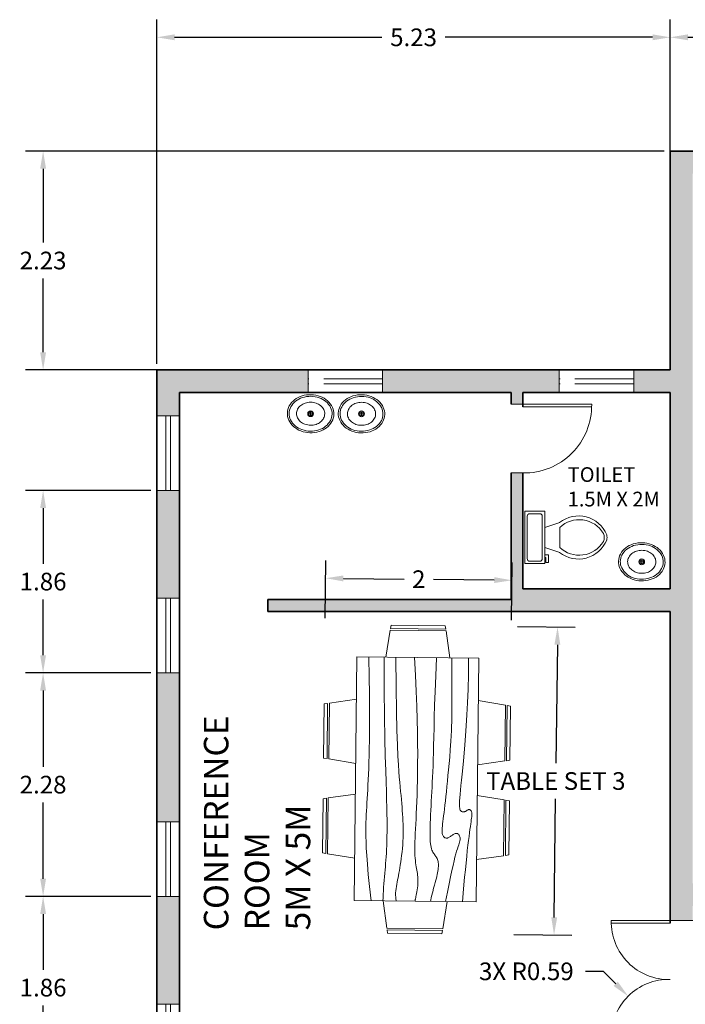
# Model space of a CAD drawing. Units: metres. Extents: x 4298.5 to 4325.2, y 2075 to 2095.8.
# Tile 18 of 35: x 4299 to 4305.8, y 2085.8 to 2095.8. Entities that reach past the tile are written whole.
import ezdxf

# ---------------------------------------------------------------- set-up
doc = ezdxf.new("R2010")
doc.units = ezdxf.units.M
doc.linetypes.add('ACAD_ISO02W100', pattern=[15, 12, -3])
for name, color, linetype, lineweight in [('A-ANNO-DIMS', 2, 'Continuous', 18), ('A-AREA-IDEN', 7, 'Continuous', 18), ('A-DOOR', 3, 'Continuous', 18), ('A-FLOR-FIXT', 15, 'Continuous', 18), ('A-FURN', 15, 'Continuous', 18), ('A-GLAZ', 4, 'Continuous', 18), ('A-GLAZ-OVHD', 4, 'ACAD_ISO02W100', 13), ('A-WALL', 7, 'Continuous', 35), ('A-WALL-PATT', 252, 'Continuous', 13)]:
    doc.layers.add(name, color=color, linetype=linetype, lineweight=lineweight)
doc.styles.get("Standard").update_dxf_attribs({"font": 'arial.ttf'})
doc.dimstyles.get("Standard").update_dxf_attribs({"dimtxt": 0.18, "dimasz": 0.18, "dimexe": 0.18, "dimexo": 0.0625, "dimgap": 0.09, "dimtad": 0, "dimtih": 1, "dimtoh": 1, "dimdec": 4, "dimzin": 0, "dimdsep": 46, "dimtxsty": 'Standard', "dimcen": 0.09, "dimadec": 0, "dimazin": 0, "dimtfac": 1, "dimtdec": 4, "dimtofl": 0, "dimtmove": 0, "dimatfit": 3, "dimfxl": 1, "dimtolj": 1, "dimtzin": 0, "dimarcsym": 0})

# ---------------------------------------------------------------- blocks, each defined once
blk = doc.blocks.new('Dining Set - 36 x 72 in.')
for p, q in [((-22, 27.5), (-22.1562, 26.50042)), ((-5.8416, 26.5), (-22.1534, 26.5)), ((-22, 27.5), (-6, 27.5)), ((-5.8437, 26.49966), (-6, 27.5)), ((6, 27.5), (5.8438, 26.50042)), ((22.1584, 26.5), (5.8466, 26.5)), ((6, 27.5), (22, 27.5)), ((22.1563, 26.49966), (22, 27.5)), ((-22.2343, 26.00059), (-23.4847, 17.99762)), ((-22.2304, 26), (-5.7608, 26)), ((-4.5152, 17.99762), (-5.7655, 25.99926)), ((5.7657, 26.00059), (4.5153, 17.99762)), ((5.7696, 26), (22.2392, 26)), ((23.4848, 17.99762), (22.2345, 25.99926)), ((36, 18), (-36, 18)), ((-36, 18), (-36, -18)), ((36, -18), (36, 18)), ((-44.0006, 8.23428), (-35.9976, 9.48474)), ((44.0006, 8.23428), (35.9976, 9.48474)), ((-45.5, 8), (-44.5004, 8.15617)), ((-45.5, 8), (-45.5, -8)), ((-44.5, -8.15843), (-44.5, 8.15338)), ((-44, 8.23041), (-44, -8.23915)), ((44, 8.23041), (44, -8.23915)), ((44.5, -8.15843), (44.5, 8.15338)), ((45.5, 8), (44.5005, 8.15617)), ((45.5, 8), (45.5, -8)), ((-44.4997, -8.15631), (-45.5, -8)), ((-35.9976, -9.48476), (-43.9993, -8.2345)), ((35.9976, -9.48476), (43.9993, -8.2345)), ((44.4997, -8.15631), (45.5, -8)), ((-36, -18), (36, -18)), ((-22.2343, -26.0006), (-23.4847, -17.99762)), ((-4.5152, -17.99762), (-5.7655, -25.99928)), ((5.7657, -26.0006), (4.5153, -17.99762)), ((23.4848, -17.99762), (22.2345, -25.99928)), ((-22.2304, -26), (-5.7608, -26)), ((5.7696, -26), (22.2392, -26)), ((-22, -27.5), (-22.1562, -26.50044)), ((-5.8416, -26.5), (-22.1534, -26.5)), ((-22, -27.5), (-6, -27.5)), ((-5.8437, -26.49967), (-6, -27.5)), ((6, -27.5), (5.8438, -26.50044)), ((22.1584, -26.5), (5.8466, -26.5)), ((6, -27.5), (22, -27.5)), ((22.1563, -26.49967), (22, -27.5))]:
    blk.add_line(p, q)
for points in [[(-36, 15), (-31.1772, 14.97754), (-26.8079, 14.91406), (-22.8538, 14.81543), (-19.276, 14.6875), (-16.0362, 14.53613), (-13.0957, 14.36718), (-10.4159, 14.18652), (-7.9583, 14), (-5.6904, 13.81315), (-3.6035, 13.63021), (-1.6954, 13.45508), (0.0365, 13.29166), (1.5945, 13.14388), (2.9811, 13.01562), (4.1988, 12.9108), (5.25, 12.83333), (6.1393, 12.78613), (6.8802, 12.76823), (7.4883, 12.77767), (7.9792, 12.8125), (8.3685, 12.87077), (8.6719, 12.95052), (8.9049, 13.0498), (9.0833, 13.16666), (9.2205, 13.29899), (9.3216, 13.44401), (9.3895, 13.59879), (9.4271, 13.76041), (9.4373, 13.92594), (9.4232, 14.09245), (9.3875, 14.257), (9.3333, 14.41666), (9.2638, 14.56917), (9.1836, 14.71484), (9.0975, 14.85465), (9.0104, 14.98958), (8.9272, 15.1206), (8.8529, 15.2487), (8.7922, 15.37483), (8.75, 15.5), (8.7305, 15.62467), (8.7344, 15.74739), (8.7617, 15.86621), (8.8125, 15.97916), (8.8867, 16.08431), (8.9844, 16.17968), (9.1055, 16.26334), (9.25, 16.33333), (9.4189, 16.38802), (9.6172, 16.42708), (9.8506, 16.45052), (10.125, 16.45833), (10.4463, 16.45052), (10.8203, 16.42708), (11.2529, 16.38802), (11.75, 16.33333), (12.3184, 16.26318), (12.9694, 16.17838), (13.7151, 16.07991), (14.5677, 15.96875), (15.5395, 15.84586), (16.6426, 15.71224), (17.8893, 15.56884), (19.2917, 15.41666), (20.859, 15.25667), (22.5879, 15.08984), (24.4721, 14.91715), (26.5052, 14.73958), (28.6809, 14.5581), (30.9929, 14.3737), (33.4347, 14.18733), (36, 14)], [(-36, 10), (-28.9766, 10.14274), (-23.1725, 10.20442), (-18.4241, 10.19775), (-14.5677, 10.13541), (-11.4399, 10.03011), (-8.877, 9.89453), (-6.7154, 9.74137), (-4.7917, 9.58333), (-2.9698, 9.43082), (-1.2246, 9.28515), (0.4415, 9.14534), (2.026, 9.01041), (3.5266, 8.87939), (4.9408, 8.7513), (6.266, 8.62516), (7.5, 8.5), (8.6411, 8.37549), (9.6914, 8.2539), (10.6538, 8.13818), (11.5312, 8.03125), (12.3267, 7.93603), (13.043, 7.85547), (13.6831, 7.79248), (14.25, 7.75), (14.7471, 7.7303), (15.1797, 7.73307), (15.5537, 7.75732), (15.875, 7.80208), (16.1494, 7.86637), (16.3828, 7.94922), (16.5811, 8.04964), (16.75, 8.16666), (16.8944, 8.29915), (17.0143, 8.44531), (17.1089, 8.60319), (17.1771, 8.77083), (17.218, 8.94629), (17.2305, 9.1276), (17.2137, 9.31282), (17.1667, 9.5), (17.0895, 9.6875), (16.987, 9.875), (16.8649, 10.0625), (16.7292, 10.25), (16.5856, 10.4375), (16.4401, 10.625), (16.2985, 10.8125), (16.1667, 11), (16.05, 11.18733), (15.9518, 11.3737), (15.8752, 11.5581), (15.8229, 11.73958), (15.798, 11.91715), (15.8034, 12.08984), (15.842, 12.25667), (15.9167, 12.41666), (16.0295, 12.56836), (16.1784, 12.70833), (16.3605, 12.83268), (16.5729, 12.9375), (16.8127, 13.01888), (17.0768, 13.07291), (17.3625, 13.0957), (17.6667, 13.08333), (17.9894, 13.03312), (18.3418, 12.94726), (18.7382, 12.82918), (19.1927, 12.68229), (19.7195, 12.51001), (20.3327, 12.31575), (21.0465, 12.10294), (21.875, 11.875), (22.8357, 11.63354), (23.959, 11.37304), (25.2786, 11.08618), (26.8282, 10.76562), (28.6414, 10.40405), (30.752, 9.99414), (33.1936, 9.52856), (36, 9)], [(-36, 5.5), (-30.7157, 5.3348), (-26.069, 5.20963), (-21.9946, 5.11767), (-18.4271, 5.05208), (-15.3009, 5.00602), (-12.5508, 4.97265), (-10.1112, 4.94515), (-7.9167, 4.91666), (-5.909, 4.88167), (-4.0586, 4.83984), (-2.3429, 4.79215), (-0.7396, 4.73958), (0.7739, 4.6831), (2.22, 4.6237), (3.6213, 4.56233), (5, 4.5), (6.373, 4.43782), (7.7344, 4.3776), (9.0723, 4.32129), (10.375, 4.27083), (11.6309, 4.22819), (12.8281, 4.19531), (13.9551, 4.17415), (15, 4.16666), (15.954, 4.17448), (16.819, 4.19791), (17.6001, 4.23698), (18.3021, 4.29166), (18.9299, 4.36198), (19.4883, 4.44791), (19.9823, 4.54948), (20.4167, 4.66666), (20.7969, 4.79899), (21.1302, 4.94401), (21.4245, 5.09879), (21.6875, 5.26041), (21.9271, 5.42594), (22.1511, 5.59245), (22.3672, 5.757), (22.5834, 5.91666), (22.8065, 6.06868), (23.0404, 6.21093), (23.2879, 6.34147), (23.5521, 6.45833), (23.8358, 6.55957), (24.142, 6.64323), (24.4735, 6.70735), (24.8334, 6.75), (25.2235, 6.76969), (25.642, 6.76692), (26.0858, 6.74267), (26.5521, 6.69791), (27.0379, 6.63362), (27.5404, 6.55078), (28.0565, 6.45036), (28.5834, 6.33333), (29.1242, 6.19987), (29.7071, 6.04687), (30.3661, 5.87044), (31.1354, 5.66666), (32.0493, 5.43164), (33.142, 5.16146), (34.4475, 4.85221), (36, 4.5)], [(-36, -1), (-30.7915, -0.6591), (-26.0195, -0.38216), (-21.6519, -0.16284), (-17.6563, 0.00521), (-14.0005, 0.12833), (-10.6523, 0.21289), (-7.5796, 0.26522), (-4.75, 0.29166), (-2.134, 0.29793), (0.2878, 0.28711), (2.5317, 0.26163), (4.6146, 0.22396), (6.5529, 0.17651), (8.3633, 0.12174), (10.0623, 0.06209), (11.6667, 0), (13.1899, -0.06201), (14.6341, -0.1211), (15.9982, -0.17432), (17.2813, -0.21875), (18.4823, -0.25147), (19.6003, -0.26953), (20.6343, -0.27002), (21.5834, -0.25), (22.4481, -0.20768), (23.2357, -0.14584), (23.9549, -0.06836), (24.6146, 0.02083), (25.2235, 0.11784), (25.7904, 0.21875), (26.3241, 0.31966), (26.8334, 0.41666), (27.3265, 0.50618), (27.8099, 0.58593), (28.2894, 0.65397), (28.7709, 0.70833), (29.2601, 0.74707), (29.763, 0.76823), (30.2855, 0.76985), (30.8334, 0.75), (31.4088, 0.70784), (31.9994, 0.64713), (32.589, 0.57275), (33.1615, 0.48958), (33.7008, 0.4025), (34.1908, 0.3164), (34.6153, 0.23616), (34.9584, 0.16666), (35.2099, 0.11165), (35.3848, 0.07031), (35.504, 0.04069), (35.5886, 0.02083), (35.6594, 0.00879), (35.7377, 0.0026), (35.8442, 0.00032), (36, 0)], [(-36, -6.5), (-27.1843, -6.31267), (-20.084, -6.1263), (-14.469, -5.9419), (-10.1094, -5.76042), (-6.7752, -5.58285), (-4.2363, -5.41016), (-2.2629, -5.24333), (-0.625, -5.08334), (0.8708, -4.93099), (2.2715, -4.78646), (3.5872, -4.64974), (4.8281, -4.52084), (6.0046, -4.39974), (7.127, -4.28646), (8.2053, -4.18099), (9.25, -4.08334), (10.2705, -3.99382), (11.2734, -3.91407), (12.2647, -3.84603), (13.25, -3.79167), (14.2354, -3.75293), (15.2266, -3.73177), (16.2295, -3.73015), (17.25, -3.75), (18.2912, -3.79248), (19.3451, -3.85547), (20.4009, -3.93604), (21.4479, -4.03125), (22.4754, -4.13819), (23.4727, -4.25391), (24.4289, -4.37549), (25.3334, -4.5), (26.1785, -4.62492), (26.9694, -4.74935), (27.7145, -4.87281), (28.4219, -4.99479), (29.1, -5.11483), (29.7572, -5.23242), (30.4016, -5.34709), (31.0417, -5.45834), (31.6837, -5.56437), (32.3262, -5.65821), (32.9658, -5.73153), (33.599, -5.77604), (34.2224, -5.78345), (34.8327, -5.74545), (35.4264, -5.65373), (36, -5.5)], [(-36, -10), (-26.4022, -9.81299), (-18.4675, -9.62891), (-11.9839, -9.45069), (-6.7396, -9.28125), (-2.5226, -9.12354), (0.8789, -8.98047), (3.6769, -8.85498), (6.0833, -8.75), (8.2767, -8.66765), (10.3021, -8.60677), (12.1712, -8.56543), (13.8958, -8.54167), (15.4876, -8.53353), (16.9583, -8.53907), (18.3197, -8.55632), (19.5834, -8.58334), (20.7616, -8.61841), (21.8685, -8.66081), (22.9188, -8.71004), (23.9271, -8.76563), (24.9081, -8.82707), (25.8763, -8.89388), (26.8465, -8.96558), (27.8334, -9.04167), (28.8474, -9.12118), (29.8828, -9.20117), (30.93, -9.27824), (31.9792, -9.34896), (33.0205, -9.40991), (34.0443, -9.45768), (35.0407, -9.48885), (36, -9.5)], [(-36, -14.5), (-30.0881, -14.33513), (-25.0332, -14.21224), (-20.7312, -14.12647), (-17.0781, -14.07292), (-13.97, -14.04671), (-11.3027, -14.04297), (-8.9724, -14.05681), (-6.875, -14.08334), (-4.9224, -14.11833), (-3.0905, -14.16016), (-1.3709, -14.20785), (0.2448, -14.26042), (1.7647, -14.3169), (3.1973, -14.3763), (4.5507, -14.43767), (5.8333, -14.5), (7.0554, -14.5621), (8.235, -14.62175), (9.3922, -14.67652), (10.5469, -14.72396), (11.7192, -14.76164), (12.929, -14.78711), (14.1965, -14.79794), (15.5417, -14.79167), (16.9933, -14.76424), (18.6152, -14.70508), (20.4804, -14.60197), (22.6615, -14.44271), (25.2312, -14.21509), (28.2624, -13.9069), (31.8277, -13.50594), (36, -13)]]:
    blk.add_lwpolyline(points)
blk = doc.blocks.new('Toilet - top')
for p, q in [((9.5, -6), (9.5, -2)), ((-10, -8.5), (-8, -8.5)), ((-10, -9.5), (-10, -8.5)), ((-7, -9.5), (-10, -9.5)), ((-8, -8.5), (-8, -8)), ((-7, -8), (-7, -9.5)), ((-4, -8), (-6, -14)), ((4, -8), (6, -14)), ((4, -14), (-4, -14))]:
    blk.add_line(p, q)
blk.add_lwpolyline([(10.5, -8), (10.5, 0), (-10.5, 0), (-10.5, -8)], close=True)
for points in [[(-9.5, -2), (-9.5, -6)], [(8.5, -1), (-8.5, -1)], [(-8.5, -7), (8.5, -7)]]:
    blk.add_lwpolyline(points)
for centre, radius, start, end in [((-8.62, -1.88), 0.884, 81.8699, 188.1301), ((8.62, -1.88), 0.884, 351.8699, 98.1301), ((-8.62, -6.12), 0.884, 171.8699, 278.1301), ((8.62, -6.12), 0.884, 261.8699, 8.1301), ((3.52, -21.58), 12.17, 141.4691, 247.9714), ((4.2, -21.82), 11.33, 136.3677, 238.9468), ((-3.52, -21.58), 12.17, 292.0284, 38.5307), ((-4.2, -21.82), 11.33, 301.053, 43.6321), ((0, -27.88), 4, 245.7318, 294.2682), ((0, -29), 4, 254.8605, 285.1395)]:
    blk.add_arc(centre, radius, start, end)
blk = doc.blocks.new('Sink - Oval top')
for p, q in [((-1, 0), (1, 0)), ((0, 1), (0, -1))]:
    blk.add_line(p, q)
for points in [[(-12.23, 0.39, 0.117634), (-11.46, -3.36, 0.104469), (-8.88, -6.8, 0.090016), (-5.08, -9.07, 0.08192), (-0.32, -10.02, 0.08192), (4.49, -9.38, 0.090016), (8.42, -7.36, 0.104469), (11.22, -4.09, 0.117634), (12.23, -0.39, 0.117634), (11.46, 3.36, 0.104469), (8.88, 6.8, 0.090016), (5.08, 9.07, 0.08192), (0.32, 10.02, 0.08192), (-4.49, 9.38, 0.090016), (-8.42, 7.36, 0.104469), (-11.22, 4.09, 0.117634)], [(-11.29, 0.16, 0.118622), (-10.52, -3.25, 0.104678), (-8.07, -6.36, 0.089562), (-4.54, -8.37, 0.081185), (-0.13, -9.15, 0.081185), (4.3, -8.49, 0.089562), (7.89, -6.58, 0.104678), (10.42, -3.55, 0.118622), (11.29, -0.16, 0.118622), (10.52, 3.25, 0.104678), (8.07, 6.36, 0.089562), (4.54, 8.37, 0.081185), (0.13, 9.15, 0.081185), (-4.3, 8.49, 0.089562), (-7.89, 6.58, 0.104678), (-10.42, 3.55, 0.118622)], [(-7.42, 0.08, 0.118283), (-6.91, -2.17, 0.104607), (-5.29, -4.21, 0.089718), (-2.97, -5.53, 0.081436), (-0.07, -6.04, 0.081436), (2.84, -5.59, 0.089718), (5.2, -4.33, 0.104607), (6.86, -2.32, 0.118283), (7.42, -0.08, 0.118283), (6.91, 2.17, 0.104607), (5.29, 4.21, 0.089718), (2.97, 5.53, 0.081436), (0.07, 6.04, 0.081436), (-2.84, 5.59, 0.089718), (-5.2, 4.33, 0.104607), (-6.86, 2.32, 0.118283)]]:
    blk.add_lwpolyline(points, format="xyb", close=True)
for radius in [1.5, 1]:
    blk.add_circle((0, 0), radius)
blk = doc.blocks.new('WIN-760-GLASS-HIGH')
at = {"ltscale": 0.05}
for p, q in [((0, 0.76), (0, 0)), ((0.05, 0.76), (0.05, 0))]:
    blk.add_line(p, q, dxfattribs=at)
blk = doc.blocks.new('WIN-760-GLASS')
for p, q in [((0, 0.76), (0, 0)), ((0.05, 0.76), (0.05, 0))]:
    blk.add_line(p, q)
blk = doc.blocks.new('DOOR-700-LEAF')
for p, q in [((0.675, 0), (0.675, 0.7)), ((0.7, 0), (0.7, 0.7))]:
    blk.add_line(p, q)
blk.add_arc((0.688, 0.012), 0.688, 88.9584, 181.0416)
blk = doc.blocks.new('DOOR-600-LEAF')
for p, q in [((0, 0), (0, 0.6)), ((0.025, 0), (0.025, 0.6))]:
    blk.add_line(p, q)
blk.add_arc((0.013, 0.013), 0.588, 358.7811, 91.2189)
blk = doc.blocks.new('*D45')
at = {"layer": 'A-ANNO-DIMS', "color": 0, "lineweight": -2, "transparency": 16777216}
for p, q in [((4304.104, 2089.633), (4304.693, 2089.627)), ((4304.511, 2089.449), (4304.497, 2088.243)), ((4304.479, 2086.671), (4304.493, 2087.877)), ((4304.069, 2086.495), (4304.657, 2086.489))]:
    blk.add_line(p, q, dxfattribs=at)
at = {"layer": 'A-ANNO-DIMS', "color": 0, "transparency": 16777216}
for points in [[(4304.481, 2089.449), (4304.541, 2089.448), (4304.513, 2089.629)], [(4304.449, 2086.671), (4304.509, 2086.67), (4304.477, 2086.491)]]:
    blk.add_solid(points, dxfattribs=at)
at = {"layer": 'Defpoints', "color": 0, "transparency": 16777216}
for p in [(4304.042, 2089.634), (4304.006, 2086.496), (4304.477, 2086.491)]:
    blk.add_point(p, dxfattribs=at)
at = {"layer": 'A-ANNO-DIMS', "color": 0, "transparency": 16777216, "insert": (4304.495, 2088.06), "char_height": 0.18, "attachment_point": 5}
blk.add_mtext('\\A1;TABLE SET 3', dxfattribs=at)
blk = doc.blocks.new('*D46')
at = {"layer": 'A-ANNO-DIMS', "color": 0, "lineweight": -2, "transparency": 16777216}
for p, q in [((4302.146, 2089.718), (4302.153, 2090.306)), ((4304.043, 2089.697), (4304.049, 2090.285)), ((4302.331, 2090.124), (4302.949, 2090.117)), ((4303.867, 2090.107), (4303.249, 2090.114))]:
    blk.add_line(p, q, dxfattribs=at)
at = {"layer": 'A-ANNO-DIMS', "color": 0, "transparency": 16777216}
for points in [[(4302.331, 2090.154), (4302.33, 2090.094), (4302.151, 2090.126)], [(4303.868, 2090.137), (4303.867, 2090.077), (4304.047, 2090.105)]]:
    blk.add_solid(points, dxfattribs=at)
at = {"layer": 'Defpoints', "color": 0, "transparency": 16777216}
for p in [(4304.047, 2090.105), (4302.145, 2089.656), (4304.042, 2089.634)]:
    blk.add_point(p, dxfattribs=at)
at = {"layer": 'A-ANNO-DIMS', "color": 0, "transparency": 16777216, "insert": (4303.099, 2090.116), "char_height": 0.18, "attachment_point": 5}
blk.add_mtext('\\A1;2', dxfattribs=at)
blk = doc.blocks.new('*D49')
at = {"layer": 'A-ANNO-DIMS', "color": 0, "lineweight": -2, "transparency": 16777216}
for p, q in [((4300.431, 2092.311), (4300.431, 2095.817)), ((4305.661, 2092.311), (4305.661, 2095.817)), ((4300.611, 2095.637), (4302.722, 2095.637)), ((4305.481, 2095.637), (4303.369, 2095.637))]:
    blk.add_line(p, q, dxfattribs=at)
at = {"layer": 'A-ANNO-DIMS', "color": 0, "transparency": 16777216}
for points in [[(4300.611, 2095.667), (4300.611, 2095.607), (4300.431, 2095.637)], [(4305.481, 2095.667), (4305.481, 2095.607), (4305.661, 2095.637)]]:
    blk.add_solid(points, dxfattribs=at)
at = {"layer": 'Defpoints', "color": 0, "transparency": 16777216}
for p in [(4305.661, 2095.637), (4300.431, 2092.248), (4305.661, 2092.248)]:
    blk.add_point(p, dxfattribs=at)
at = {"layer": 'A-ANNO-DIMS', "color": 0, "transparency": 16777216, "insert": (4303.046, 2095.637), "char_height": 0.18, "attachment_point": 5}
blk.add_mtext('\\A1;5.23', dxfattribs=at)
blk = doc.blocks.new('*D50')
at = {"layer": 'A-ANNO-DIMS', "color": 0, "lineweight": -2, "transparency": 16777216}
for p, q in [((4305.661, 2094.541), (4305.661, 2095.817)), ((4310.121, 2094.541), (4310.121, 2095.817)), ((4305.841, 2095.637), (4307.563, 2095.637)), ((4309.941, 2095.637), (4308.218, 2095.637))]:
    blk.add_line(p, q, dxfattribs=at)
at = {"layer": 'A-ANNO-DIMS', "color": 0, "transparency": 16777216}
for points in [[(4305.841, 2095.667), (4305.841, 2095.607), (4305.661, 2095.637)], [(4309.941, 2095.667), (4309.941, 2095.607), (4310.121, 2095.637)]]:
    blk.add_solid(points, dxfattribs=at)
at = {"layer": 'Defpoints', "color": 0, "transparency": 16777216}
for p in [(4310.121, 2095.637), (4305.661, 2094.478), (4310.121, 2094.478)]:
    blk.add_point(p, dxfattribs=at)
at = {"layer": 'A-ANNO-DIMS', "color": 0, "transparency": 16777216, "insert": (4307.891, 2095.637), "char_height": 0.18, "attachment_point": 5}
blk.add_mtext('\\A1;4.46', dxfattribs=at)
blk = doc.blocks.new('*D52')
at = {"layer": 'A-ANNO-DIMS', "color": 0, "lineweight": -2, "transparency": 16777216}
for p, q in [((4305.598, 2094.478), (4299.092, 2094.478)), ((4299.272, 2094.298), (4299.272, 2093.545)), ((4299.272, 2092.428), (4299.272, 2093.181)), ((4305.598, 2092.248), (4299.092, 2092.248))]:
    blk.add_line(p, q, dxfattribs=at)
at = {"layer": 'A-ANNO-DIMS', "color": 0, "transparency": 16777216}
for points in [[(4299.242, 2094.298), (4299.302, 2094.298), (4299.272, 2094.478)], [(4299.242, 2092.428), (4299.302, 2092.428), (4299.272, 2092.248)]]:
    blk.add_solid(points, dxfattribs=at)
at = {"layer": 'Defpoints', "color": 0, "transparency": 16777216}
for p in [(4299.272, 2094.478), (4305.661, 2094.478), (4305.661, 2092.248)]:
    blk.add_point(p, dxfattribs=at)
at = {"layer": 'A-ANNO-DIMS', "color": 0, "transparency": 16777216, "insert": (4299.272, 2093.363), "char_height": 0.18, "attachment_point": 5}
blk.add_mtext('\\A1;2.23', dxfattribs=at)
blk = doc.blocks.new('*D75')
at = {"layer": 'A-ANNO-DIMS', "color": 0, "lineweight": -2, "transparency": 16777216}
for p, q in [((4300.368, 2086.884), (4299.092, 2086.884)), ((4299.272, 2086.704), (4299.272, 2086.137)), ((4299.272, 2085.205), (4299.272, 2085.773)), ((4300.368, 2085.025), (4299.092, 2085.025))]:
    blk.add_line(p, q, dxfattribs=at)
at = {"layer": 'A-ANNO-DIMS', "color": 0, "transparency": 16777216}
for points in [[(4299.242, 2086.704), (4299.302, 2086.704), (4299.272, 2086.884)], [(4299.242, 2085.205), (4299.302, 2085.205), (4299.272, 2085.025)]]:
    blk.add_solid(points, dxfattribs=at)
at = {"layer": 'Defpoints', "color": 0, "transparency": 16777216}
for p in [(4299.272, 2086.884), (4300.431, 2086.884), (4300.431, 2085.025)]:
    blk.add_point(p, dxfattribs=at)
at = {"layer": 'A-ANNO-DIMS', "color": 0, "transparency": 16777216, "insert": (4299.272, 2085.955), "char_height": 0.18, "attachment_point": 5}
blk.add_mtext('\\A1;1.86', dxfattribs=at)
blk = doc.blocks.new('*D76')
at = {"layer": 'A-ANNO-DIMS', "color": 0, "lineweight": -2, "transparency": 16777216}
for p, q in [((4300.368, 2089.162), (4299.092, 2089.162)), ((4299.272, 2088.982), (4299.272, 2088.205)), ((4299.272, 2087.064), (4299.272, 2087.841)), ((4300.368, 2086.884), (4299.092, 2086.884))]:
    blk.add_line(p, q, dxfattribs=at)
at = {"layer": 'A-ANNO-DIMS', "color": 0, "transparency": 16777216}
for points in [[(4299.242, 2088.982), (4299.302, 2088.982), (4299.272, 2089.162)], [(4299.242, 2087.064), (4299.302, 2087.064), (4299.272, 2086.884)]]:
    blk.add_solid(points, dxfattribs=at)
at = {"layer": 'Defpoints', "color": 0, "transparency": 16777216}
for p in [(4299.272, 2089.162), (4300.431, 2089.162), (4300.431, 2086.884)]:
    blk.add_point(p, dxfattribs=at)
at = {"layer": 'A-ANNO-DIMS', "color": 0, "transparency": 16777216, "insert": (4299.272, 2088.023), "char_height": 0.18, "attachment_point": 5}
blk.add_mtext('\\A1;2.28', dxfattribs=at)
blk = doc.blocks.new('*D77')
at = {"layer": 'A-ANNO-DIMS', "color": 0, "lineweight": -2, "transparency": 16777216}
for p, q in [((4300.368, 2091.021), (4299.092, 2091.021)), ((4299.272, 2090.841), (4299.272, 2090.273)), ((4299.272, 2089.342), (4299.272, 2089.91)), ((4300.368, 2089.162), (4299.092, 2089.162))]:
    blk.add_line(p, q, dxfattribs=at)
at = {"layer": 'A-ANNO-DIMS', "color": 0, "transparency": 16777216}
for points in [[(4299.242, 2090.841), (4299.302, 2090.841), (4299.272, 2091.021)], [(4299.242, 2089.342), (4299.302, 2089.342), (4299.272, 2089.162)]]:
    blk.add_solid(points, dxfattribs=at)
at = {"layer": 'Defpoints', "color": 0, "transparency": 16777216}
for p in [(4299.272, 2091.021), (4300.431, 2091.021), (4300.431, 2089.162)]:
    blk.add_point(p, dxfattribs=at)
at = {"layer": 'A-ANNO-DIMS', "color": 0, "transparency": 16777216, "insert": (4299.272, 2090.092), "char_height": 0.18, "attachment_point": 5}
blk.add_mtext('\\A1;1.86', dxfattribs=at)
blk = doc.blocks.new('*D82')
at = {"layer": 'A-ANNO-DIMS', "color": 0, "lineweight": -2, "transparency": 16777216}
for p, q in [((4304.798, 2086.121), (4304.978, 2086.121)), ((4304.978, 2086.121), (4305.106, 2085.994)), ((4305.648, 2085.361), (4305.648, 2085.541)), ((4305.558, 2085.451), (4305.738, 2085.451))]:
    blk.add_line(p, q, dxfattribs=at)
at = {"layer": 'A-ANNO-DIMS', "color": 0, "transparency": 16777216}
blk.add_solid([(4305.127, 2086.015), (4305.084, 2085.972), (4305.233, 2085.866)], dxfattribs=at)
at = {"layer": 'Defpoints', "color": 0, "transparency": 16777216}
for p in [(4305.233, 2085.866), (4305.648, 2085.451)]:
    blk.add_point(p, dxfattribs=at)
at = {"layer": 'A-ANNO-DIMS', "color": 0, "transparency": 16777216, "insert": (4304.195, 2086.121), "char_height": 0.18, "attachment_point": 5}
blk.add_mtext('\\A1;3X R0.59', dxfattribs=at)

msp = doc.modelspace()

# ---------------------------------------------------------------- hatches: boundary and pattern name
at = {"layer": 'A-WALL-PATT'}
h = msp.add_hatch(color=256, dxfattribs=at)
h.dxf.hatch_style = 1
h.paths.add_polyline_path([(4308.7606, 2094.4781), (4308.1606, 2094.4781), (4307.4606, 2094.4781), (4307.4606, 2094.2481), (4308.2706, 2094.2481), (4308.2706, 2094.1281), (4308.3906, 2094.1281), (4308.3906, 2094.2481), (4308.7606, 2094.2481)])
h.paths.add_polyline_path([(4310.1206, 2094.4781), (4309.5206, 2094.4781), (4309.5206, 2094.2481), (4309.8906, 2094.2481), (4309.8906, 2092.2481), (4308.3906, 2092.2481), (4308.3906, 2093.4281), (4308.2706, 2093.4281), (4308.2706, 2092.0181), (4309.8906, 2092.0181), (4309.8906, 2087.0181), (4309.7706, 2087.0181), (4309.7706, 2086.7881), (4309.8906, 2086.7881), (4311.9406, 2086.7881), (4311.9406, 2087.0181), (4310.1206, 2087.0181), (4310.1206, 2089.0181), (4310.2406, 2089.0181), (4310.2406, 2089.1381), (4310.1206, 2089.1381), (4310.1206, 2092.0181), (4310.3078, 2092.0181), (4310.3078, 2092.2481), (4310.1206, 2092.2481)])
h.paths.add_polyline_path([(4311.7406, 2092.2481), (4311.0678, 2092.2481), (4311.0678, 2092.0181), (4311.7406, 2092.0181)], flags=17)
h.paths.add_polyline_path([(4313.1733, 2092.2481), (4312.5006, 2092.2481), (4312.5006, 2092.0181), (4313.1733, 2092.0181)])
h.paths.add_polyline_path([(4314.5378, 2092.2481), (4314.1206, 2092.2481), (4313.9333, 2092.2481), (4313.9333, 2092.0181), (4314.1206, 2092.0181), (4314.1206, 2087.0181), (4314.0006, 2087.0181), (4314.0006, 2086.7881), (4314.1206, 2086.7881), (4315.5718, 2086.7881), (4315.5718, 2087.0181), (4314.3506, 2087.0181), (4314.3506, 2092.0181), (4314.5378, 2092.0181)])
h.paths.add_polyline_path([(4315.9706, 2092.2481), (4315.2978, 2092.2481), (4315.2978, 2092.0181), (4315.9706, 2092.0181)])
h.paths.add_polyline_path([(4317.4033, 2092.2481), (4316.7306, 2092.2481), (4316.7306, 2092.0181), (4317.4033, 2092.0181)])
h.paths.add_polyline_path([(4318.9506, 2092.2481), (4318.3506, 2092.2481), (4318.1633, 2092.2481), (4318.1633, 2092.0181), (4318.3506, 2092.0181), (4318.3506, 2091.8981), (4318.5806, 2091.8981), (4318.5806, 2092.0181), (4318.9506, 2092.0181)])
h.paths.add_polyline_path([(4321.0106, 2092.2481), (4319.7106, 2092.2481), (4319.7106, 2092.0181), (4320.0806, 2092.0181), (4320.0806, 2090.0181), (4318.5806, 2090.0181), (4318.5806, 2091.1981), (4318.3506, 2091.1981), (4318.3506, 2090.0181), (4318.3506, 2087.0181), (4318.2306, 2087.0181), (4318.2306, 2086.7881), (4318.3506, 2086.7881), (4318.3506, 2086.3081), (4318.5806, 2086.3081), (4318.5806, 2089.7881), (4321.7806, 2089.7881), (4321.7806, 2090.0181), (4320.2006, 2090.0181), (4320.2006, 2092.0181), (4321.0106, 2092.0181)])
h.paths.add_polyline_path([(4322.8106, 2092.2481), (4321.7706, 2092.2481), (4321.7706, 2092.0181), (4322.5806, 2092.0181), (4322.5806, 2091.2831), (4322.8106, 2091.2831)])
h.paths.add_polyline_path([(4322.8106, 2090.5231), (4322.5806, 2090.5231), (4322.5806, 2089.7881), (4322.5806, 2089.5254), (4322.8106, 2089.5254), (4322.8106, 2090.0181)])
h.paths.add_polyline_path([(4322.8106, 2088.7654), (4322.5806, 2088.7654), (4322.5806, 2087.6681), (4322.8106, 2087.6681)])
h.paths.add_polyline_path([(4322.8106, 2086.9081), (4322.5806, 2086.9081), (4322.5806, 2085.8107), (4322.8106, 2085.8107)])
h.paths.add_polyline_path([(4322.8106, 2085.0507), (4322.5806, 2085.0507), (4322.5806, 2084.7881), (4318.5806, 2084.7881), (4318.5806, 2085.0581), (4318.5806, 2085.4081), (4318.3506, 2085.4081), (4318.3506, 2084.5581), (4318.3506, 2080.8581), (4318.4706, 2080.8581), (4318.4706, 2082.3281), (4319.2606, 2082.3281), (4319.2606, 2082.5581), (4318.5806, 2082.5581), (4318.5806, 2084.5581), (4320.0806, 2084.5581), (4320.0806, 2083.9381), (4320.3106, 2083.9381), (4320.3106, 2084.5581), (4322.8106, 2084.5581)])
h.paths.add_polyline_path([(4320.3106, 2083.1781), (4320.0806, 2083.1781), (4320.0806, 2082.5581), (4319.9606, 2082.5581), (4319.9606, 2082.3281), (4320.0806, 2082.3281), (4320.0806, 2081.5731), (4320.3106, 2081.5731)], flags=17)
h.paths.add_polyline_path([(4320.3106, 2080.8131), (4320.0806, 2080.8131), (4320.0806, 2080.0581), (4318.4286, 2080.0581), (4318.4286, 2079.8281), (4320.3106, 2079.8281)])
h.paths.add_polyline_path([(4317.3506, 2085.2881), (4316.5718, 2085.2881), (4316.5718, 2085.0581), (4317.3506, 2085.0581)])
h.paths.add_polyline_path([(4315.5718, 2085.2881), (4314.8434, 2085.2881), (4314.8434, 2085.0581), (4315.5718, 2085.0581)])
h.paths.add_polyline_path([(4313.8434, 2085.2881), (4312.9406, 2085.2881), (4312.9406, 2085.0581), (4313.8434, 2085.0581)])
h.paths.add_polyline_path([(4311.9406, 2085.2881), (4311.4406, 2085.2881), (4311.4406, 2085.0581), (4311.9406, 2085.0581)])
h.paths.add_polyline_path([(4317.3306, 2087.0181), (4316.5718, 2087.0181), (4316.5718, 2086.7881), (4317.3306, 2086.7881)])
h.paths.add_polyline_path([(4313.1006, 2089.1381), (4311.1406, 2089.1381), (4311.1406, 2089.0181), (4312.9806, 2089.0181), (4312.9806, 2087.0181), (4312.9406, 2087.0181), (4312.9406, 2086.7881), (4313.1006, 2086.7881), (4313.1006, 2087.0181)])
h.paths.add_polyline_path([(4307.5515, 2087.0181), (4305.8906, 2087.0181), (4305.8906, 2092.2481), (4305.8906, 2094.2481), (4306.7006, 2094.2481), (4306.7006, 2094.4781), (4305.6606, 2094.4781), (4305.6606, 2092.2481), (4305.2906, 2092.2481), (4305.2906, 2092.0181), (4305.6606, 2092.0181), (4305.6606, 2090.0181), (4304.1606, 2090.0181), (4304.1606, 2091.1981), (4304.0406, 2091.1981), (4304.0406, 2089.9081), (4301.5606, 2089.9081), (4301.5606, 2089.7881), (4304.0406, 2089.7881), (4305.6606, 2089.7881), (4305.6606, 2086.6381), (4305.8906, 2086.6381), (4305.8906, 2086.7881), (4307.5515, 2086.7881)])
h.paths.add_polyline_path([(4307.5515, 2085.2881), (4305.8906, 2085.2881), (4305.8906, 2085.4381), (4305.6606, 2085.4381), (4305.6606, 2084.7881), (4305.2906, 2084.7881), (4305.2906, 2084.5581), (4305.6606, 2084.5581), (4305.6606, 2084.02), (4305.8906, 2084.02), (4305.8906, 2084.5581), (4305.8906, 2085.0581), (4307.5515, 2085.0581)])
h.paths.add_polyline_path([(4310.2406, 2085.2881), (4308.5515, 2085.2881), (4308.5515, 2085.0581), (4310.2406, 2085.0581)])
h.paths.add_polyline_path([(4317.4286, 2080.0581), (4316.5718, 2080.0581), (4316.5718, 2079.8281), (4317.4286, 2079.8281)])
h.paths.add_polyline_path([(4315.5718, 2080.0581), (4314.8434, 2080.0581), (4314.8434, 2079.8281), (4315.5718, 2079.8281)])
h.paths.add_polyline_path([(4313.8434, 2080.0581), (4312.9406, 2080.0581), (4312.9406, 2079.8281), (4313.8434, 2079.8281)])
h.paths.add_polyline_path([(4311.9406, 2080.0581), (4311.4406, 2080.0581), (4311.4406, 2079.8281), (4311.9406, 2079.8281)])
h.paths.add_polyline_path([(4310.2406, 2080.0581), (4310.1206, 2080.0581), (4310.1206, 2084.0381), (4309.8906, 2084.0381), (4309.8906, 2080.0581), (4309.1606, 2080.0581), (4309.1606, 2079.8281), (4310.2406, 2079.8281)])
h.paths.add_polyline_path([(4308.1606, 2080.0581), (4307.5106, 2080.0581), (4307.5106, 2080.1781), (4307.3906, 2080.1781), (4307.3906, 2080.0581), (4305.8906, 2080.0581), (4305.8906, 2080.567), (4305.6606, 2080.567), (4305.6606, 2079.8281), (4308.1606, 2079.8281)])
h.paths.add_polyline_path([(4307.5106, 2081.9381), (4309.0906, 2081.9381), (4309.0906, 2082.0581), (4305.8906, 2082.0581), (4305.8906, 2083.26), (4305.6606, 2083.26), (4305.6606, 2081.327), (4305.8906, 2081.327), (4305.8906, 2081.9381), (4307.3906, 2081.9381), (4307.3906, 2080.8781), (4307.5106, 2080.8781)])
h.paths.add_polyline_path([(4304.5306, 2084.7881), (4302.7306, 2084.7881), (4302.7306, 2084.5581), (4304.5306, 2084.5581)])
h.paths.add_polyline_path([(4301.9706, 2084.7881), (4300.6606, 2084.7881), (4300.6606, 2085.0249), (4300.4306, 2085.0249), (4300.4306, 2084.5581), (4301.9706, 2084.5581)])
h.paths.add_polyline_path([(4300.6606, 2086.8843), (4300.4306, 2086.8843), (4300.4306, 2085.7849), (4300.6606, 2085.7849)])
h.paths.add_polyline_path([(4300.6606, 2089.1618), (4300.4306, 2089.1618), (4300.4306, 2087.6443), (4300.6606, 2087.6443)])
h.paths.add_polyline_path([(4300.6606, 2091.0212), (4300.4306, 2091.0212), (4300.4306, 2089.9218), (4300.6606, 2089.9218)])
h.paths.add_polyline_path([(4300.6606, 2092.0181), (4301.9706, 2092.0181), (4301.9706, 2092.2481), (4300.4306, 2092.2481), (4300.4306, 2091.7812), (4300.6606, 2091.7812)])
h.paths.add_polyline_path([(4304.5306, 2092.2481), (4302.7306, 2092.2481), (4302.7306, 2092.0181), (4304.0406, 2092.0181), (4304.0406, 2091.8981), (4304.1606, 2091.8981), (4304.1606, 2092.0181), (4304.5306, 2092.0181)], flags=17)

# ---------------------------------------------------------------- linework, layer by layer
at = {"layer": 'A-DOOR'}
for p, q in [((4304.1606, 2091.8981), (4304.0406, 2091.8981)), ((4304.1606, 2091.1981), (4304.0406, 2091.1981)), ((4305.8906, 2086.6381), (4305.6606, 2086.6381))]:
    msp.add_line(p, q, dxfattribs=at)
at = {"layer": 'A-GLAZ'}
for p, q in [((4301.9706, 2092.0181), (4301.9706, 2092.2481)), ((4302.7306, 2092.0181), (4302.7306, 2092.2481)), ((4304.5306, 2092.0181), (4304.5306, 2092.2481)), ((4305.2906, 2092.0181), (4305.2906, 2092.2481)), ((4300.6606, 2091.7812), (4300.4306, 2091.7812)), ((4300.6606, 2091.0212), (4300.4306, 2091.0212)), ((4300.6606, 2089.9218), (4300.4306, 2089.9218)), ((4300.6606, 2089.1618), (4300.4306, 2089.1618)), ((4300.6606, 2087.6443), (4300.4306, 2087.6443)), ((4300.6606, 2086.8843), (4300.4306, 2086.8843)), ((4300.6606, 2085.7849), (4300.4306, 2085.7849))]:
    msp.add_line(p, q, dxfattribs=at)
at = {"layer": 'A-WALL'}
for p, q in [((4308.3906, 2094.4781), (4305.6606, 2094.4781)), ((4305.6606, 2092.2481), (4305.6606, 2094.4781)), ((4305.6606, 2092.2481), (4300.4306, 2092.2481)), ((4300.4306, 2084.5581), (4300.4306, 2092.2481)), ((4300.6606, 2089.7881), (4300.6606, 2092.0181)), ((4304.0406, 2092.0181), (4300.6606, 2092.0181)), ((4304.0406, 2092.0181), (4304.0406, 2091.8981)), ((4305.6606, 2092.0181), (4304.1606, 2092.0181)), ((4304.1606, 2092.0181), (4304.1606, 2091.8731)), ((4305.6606, 2092.0181), (4305.6606, 2090.0181)), ((4304.0406, 2091.1981), (4304.0406, 2089.9081)), ((4304.1606, 2091.1981), (4304.1606, 2090.0181)), ((4305.6606, 2090.0181), (4304.1606, 2090.0181)), ((4304.0406, 2089.9081), (4301.5606, 2089.9081)), ((4301.5606, 2089.7881), (4301.5606, 2089.9081)), ((4300.6606, 2084.7881), (4300.6606, 2089.7881)), ((4304.0406, 2089.7881), (4301.5606, 2089.7881)), ((4305.6606, 2089.7881), (4304.0406, 2089.7881)), ((4305.6606, 2089.7881), (4305.6606, 2086.6131))]:
    msp.add_line(p, q, dxfattribs=at)

# ---------------------------------------------------------------- block references
at = {"layer": 'A-DOOR', "extrusion": (0, 0, -1), "zscale": -1}
for name, p, rotation in [('DOOR-700-LEAF', (-4304.1606, 2091.198), 89.99999999999999), ('DOOR-600-LEAF', (-4305.6606, 2086.6381), 269.9999999998974)]:
    msp.add_blockref(name, p, dxfattribs=dict(at, rotation=rotation))
at = {"layer": 'A-DOOR', "rotation": 89.9999999966095}
msp.add_blockref('DOOR-600-LEAF', (4305.6606, 2085.4381), dxfattribs=at)
at = {"layer": 'A-FLOR-FIXT', "xscale": 0.0193818050953029, "yscale": 0.0193818050953029, "zscale": 0.0193818050953029}
for p in [(4301.9971, 2091.8019), (4302.5157, 2091.801), (4305.3708, 2090.2932)]:
    msp.add_blockref('Sink - Oval top', p, dxfattribs=at)
at = {"layer": 'A-FLOR-FIXT', "xscale": 0.0254, "yscale": 0.0254, "zscale": 0.0254, "rotation": 90.00015040587188}
msp.add_blockref('Toilet - top', (4304.1788, 2090.5415), dxfattribs=at)
at = {"layer": 'A-FURN', "xscale": 0.034484439092578, "yscale": 0.034484439092578, "zscale": 0.034484439092578, "rotation": 269.3494212219322}
msp.add_blockref('Dining Set - 36 x 72 in.', (4303.0758, 2088.0759), dxfattribs=at)
at = {"layer": 'A-GLAZ'}
for p in [(4300.5206, 2091.0212), (4300.5206, 2089.1618), (4300.5206, 2086.8843), (4300.5206, 2085.0249)]:
    msp.add_blockref('WIN-760-GLASS', p, dxfattribs=at)
at = {"layer": 'A-GLAZ-OVHD', "rotation": 269.9999999999317}
for p in [(4301.9706, 2092.1581), (4304.5306, 2092.1581)]:
    msp.add_blockref('WIN-760-GLASS-HIGH', p, dxfattribs=at)

# ---------------------------------------------------------------- texts
at = {"layer": 'A-AREA-IDEN', "insert": (4304.6161, 2091.2575), "char_height": 0.15, "attachment_point": 1}
msp.add_mtext_dynamic_manual_height_columns('TOILET\\P1.5M X 2M', width=2.22034, gutter_width=12.5, heights=[0], dxfattribs=at)
at = {"layer": 'A-AREA-IDEN', "insert": (4300.9098, 2086.5385), "char_height": 0.25, "attachment_point": 1, "rotation": 90}
msp.add_mtext_dynamic_manual_height_columns('CONFERENCE ROOM\\P5M X 5M', width=2.22034, gutter_width=12.5, heights=[0], dxfattribs=at)

# ---------------------------------------------------------------- dimensions: what is measured, and where the dimension line sits
at = {"layer": 'A-ANNO-DIMS'}
for base, p1, p2, picture, middle in [((4305.6606, 2095.6366), (4300.4306, 2092.2481), (4305.6606, 2092.2481), '*D49', (4303.0456, 2095.6366)), ((4310.1206, 2095.6366), (4305.6606, 2094.4781), (4310.1206, 2094.4781), '*D50', (4307.8906, 2095.6366))]:
    dim = msp.add_linear_dim(base=base, p1=p1, p2=p2, dimstyle='Standard', override={"dimdec": 2, "dimlfac": 1, "dimrnd": 0, "dimzin": 0, "dimdsep": 46, "dimlunit": 2}, dxfattribs=at)
    dim.commit()
    dim.dimension.update_dxf_attribs({"geometry": picture, "text_midpoint": middle})
for base, p1, p2, angle, override, picture, middle in [((4299.2721, 2094.4781), (4305.6606, 2092.2481), (4305.6606, 2094.4781), 90, {"dimdec": 2, "dimlfac": 1, "dimrnd": 0, "dimzin": 0, "dimdsep": 46, "dimlunit": 2}, '*D52', (4299.2721, 2093.3631)), ((4299.2721, 2091.0212), (4300.4306, 2089.1618), (4300.4306, 2091.0212), 90, {"dimdec": 2, "dimlfac": 1, "dimrnd": 0, "dimzin": 0, "dimdsep": 46, "dimlunit": 2}, '*D77', (4299.2721, 2090.0915)), ((4304.0473, 2090.1048), (4302.1454, 2089.6556), (4304.0419, 2089.6341), 359.34942, {"dimdec": 0, "dimlfac": 1, "dimrnd": 0, "dimzin": 0, "dimdsep": 46, "dimlunit": 2}, '*D46', (4303.099, 2090.1155)), ((4299.2721, 2089.1618), (4300.4306, 2086.8843), (4300.4306, 2089.1618), 90, {"dimdec": 2, "dimlfac": 1, "dimrnd": 0, "dimzin": 0, "dimdsep": 46, "dimlunit": 2}, '*D76', (4299.2721, 2088.0231)), ((4299.2721, 2086.8843), (4300.4306, 2085.0249), (4300.4306, 2086.8843), 90, {"dimdec": 2, "dimlfac": 1, "dimrnd": 0, "dimzin": 0, "dimdsep": 46, "dimlunit": 2}, '*D75', (4299.2721, 2085.9546))]:
    dim = msp.add_linear_dim(base=base, p1=p1, p2=p2, angle=angle, dimstyle='Standard', override=override, dxfattribs=at)
    dim.commit()
    dim.dimension.update_dxf_attribs({"geometry": picture, "text_midpoint": middle})
dim = msp.add_linear_dim(base=(4304.477, 2086.4908), p1=(4304.0419, 2089.6341), p2=(4304.0063, 2086.4962), angle=269.34942, text='TABLE SET <>', dimstyle='Standard', override={"dimdec": 0, "dimlfac": 1, "dimrnd": 0, "dimzin": 0, "dimdsep": 46, "dimlunit": 2}, dxfattribs=at)
dim.commit()
dim.dimension.update_dxf_attribs({"geometry": '*D45', "text_midpoint": (4304.4948, 2088.0598)})
dim = msp.add_radius_dim(center=(4305.6481, 2085.4506), mpoint=(4305.2327, 2085.8663), text='3X <>', dimstyle='Standard', override={"dimdec": 2, "dimlfac": 1, "dimrnd": 0, "dimzin": 0, "dimdsep": 46, "dimlunit": 2}, dxfattribs=at)
dim.commit()
dim.dimension.update_dxf_attribs({"geometry": '*D82', "text_midpoint": (4304.1949, 2086.1209)})

doc.saveas('drawing.dxf')
